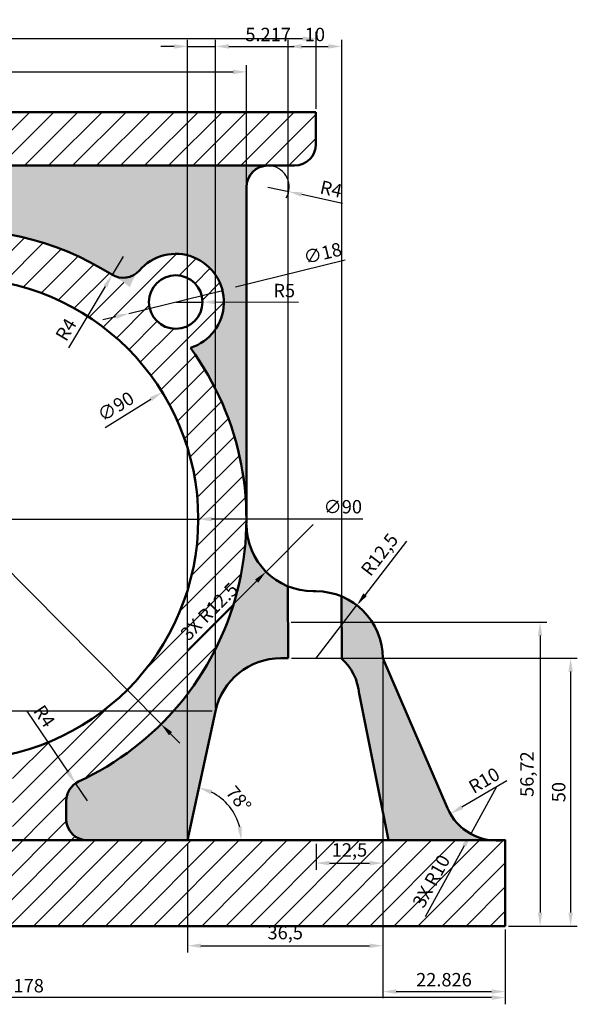
# Model space of a CAD drawing. Units: millimetres. Extents: x 2530 to 2750, y 1494 to 1677.
# Tile 2 of 2: x 2646 to 2750, y 1494 to 1677. Entities that reach past the tile are written whole.
import ezdxf

# ---------------------------------------------------------------- set-up
doc = ezdxf.new("R2010")
doc.units = ezdxf.units.MM
for name, color, linetype, lineweight in [('M-DIMS', 2, 'Continuous', 25), ('M-HATC', 8, 'Continuous', 18), ('M-OUTL', 7, 'Continuous', 50)]:
    doc.layers.add(name, color=color, linetype=linetype, lineweight=lineweight)
doc.styles.get("Standard").update_dxf_attribs({"font": 'arial.ttf'})
doc.dimstyles.new('ISO-25', dxfattribs={"dimtxt": 2.5, "dimasz": 2.5, "dimexe": 1.25, "dimexo": 0.625, "dimtad": 1, "dimtxsty": 'Standard', "dimcen": 2.5, "dimadec": 0, "dimazin": 0, "dimtfac": 1, "dimtmove": 0, "dimatfit": 3, "dimfxl": 1, "dimarcsym": 0})

# ---------------------------------------------------------------- blocks, each defined once
blk = doc.blocks.new('*D3')
at = {"layer": 'Defpoints', "color": 0, "transparency": 16777216}
for p in [(2688.41, 1667.62), (2580.41, 1646.13), (2688.41, 1646.13)]:
    blk.add_point(p, dxfattribs=at)
at = {"layer": 'M-DIMS', "color": 0, "lineweight": -2, "transparency": 16777216}
for p, q in [((2580.41, 1646.75), (2580.41, 1668.87)), ((2688.41, 1646.75), (2688.41, 1668.87)), ((2582.91, 1667.62), (2685.91, 1667.62))]:
    blk.add_line(p, q, dxfattribs=at)
at = {"layer": 'M-DIMS', "color": 0, "transparency": 16777216}
for points in [[(2582.91, 1668.04), (2582.91, 1667.2), (2580.41, 1667.62)], [(2685.91, 1668.04), (2685.91, 1667.2), (2688.41, 1667.62)]]:
    blk.add_solid(points, dxfattribs=at)
at = {"layer": 'M-DIMS', "color": 0, "transparency": 16777216, "insert": (2634.41, 1669.52), "char_height": 2.5, "attachment_point": 5}
blk.add_mtext('108', dxfattribs=at)
blk = doc.blocks.new('*D4')
at = {"layer": 'Defpoints', "color": 0, "transparency": 16777216}
for p in [(2701.41, 1673.83), (2567.41, 1660.13), (2701.41, 1660.13)]:
    blk.add_point(p, dxfattribs=at)
at = {"layer": 'M-DIMS', "color": 0, "lineweight": -2, "transparency": 16777216}
for p, q in [((2567.41, 1660.75), (2567.41, 1675.08)), ((2701.41, 1660.75), (2701.41, 1675.08)), ((2569.91, 1673.83), (2698.91, 1673.83))]:
    blk.add_line(p, q, dxfattribs=at)
at = {"layer": 'M-DIMS', "color": 0, "transparency": 16777216}
for points in [[(2569.91, 1674.25), (2569.91, 1673.41), (2567.41, 1673.83)], [(2698.91, 1674.25), (2698.91, 1673.41), (2701.41, 1673.83)]]:
    blk.add_solid(points, dxfattribs=at)
at = {"layer": 'M-DIMS', "color": 0, "transparency": 16777216, "insert": (2634.41, 1675.73), "char_height": 2.5, "attachment_point": 5}
blk.add_mtext('134', dxfattribs=at)
blk = doc.blocks.new('*D11')
at = {"layer": 'Defpoints', "color": 0, "transparency": 16777216}
for p in [(2677.41, 1524.13), (2713.91, 1524.13), (2713.91, 1504.45)]:
    blk.add_point(p, dxfattribs=at)
at = {"layer": 'M-DIMS', "color": 0, "lineweight": -2, "transparency": 16777216}
for p, q in [((2677.41, 1523.5), (2677.41, 1503.2)), ((2713.91, 1523.5), (2713.91, 1503.2)), ((2679.91, 1504.45), (2711.41, 1504.45))]:
    blk.add_line(p, q, dxfattribs=at)
at = {"layer": 'M-DIMS', "color": 0, "transparency": 16777216}
for points in [[(2679.91, 1504.86), (2679.91, 1504.03), (2677.41, 1504.45)], [(2711.41, 1504.86), (2711.41, 1504.03), (2713.91, 1504.45)]]:
    blk.add_solid(points, dxfattribs=at)
at = {"layer": 'M-DIMS', "color": 0, "transparency": 16777216, "insert": (2695.66, 1506.57), "char_height": 2.5, "attachment_point": 5}
blk.add_mtext('36,5', dxfattribs=at)
blk = doc.blocks.new('*D12')
at = {"layer": 'Defpoints', "color": 0, "transparency": 16777216}
for p in [(2696.18, 1564.85), (2736.73, 1508.13), (2743.28, 1508.13)]:
    blk.add_point(p, dxfattribs=at)
at = {"layer": 'M-DIMS', "color": 0, "lineweight": -2, "transparency": 16777216}
for p, q in [((2696.8, 1564.85), (2744.53, 1564.85)), ((2743.28, 1562.35), (2743.28, 1510.63)), ((2737.36, 1508.13), (2744.53, 1508.13))]:
    blk.add_line(p, q, dxfattribs=at)
at = {"layer": 'M-DIMS', "color": 0, "transparency": 16777216}
for points in [[(2742.86, 1562.35), (2743.69, 1562.35), (2743.28, 1564.85)], [(2742.86, 1510.63), (2743.69, 1510.63), (2743.28, 1508.13)]]:
    blk.add_solid(points, dxfattribs=at)
at = {"layer": 'M-DIMS', "color": 0, "transparency": 16777216, "insert": (2741.15, 1536.49), "char_height": 2.5, "attachment_point": 5, "rotation": 90}
blk.add_mtext('56,72', dxfattribs=at)
blk = doc.blocks.new('*D13')
at = {"layer": 'Defpoints', "color": 0, "transparency": 16777216}
for p in [(2682.63, 1548.27), (2686.45, 1528.53), (2677.41, 1524.13), (2677.41, 1524.13), (2701.41, 1524.13)]:
    blk.add_point(p, dxfattribs=at)
at = {"layer": 'M-DIMS', "color": 0, "lineweight": -2, "transparency": 16777216}
blk.add_arc((2677.41, 1524.13), 10.05, 14.2844, 63.521, dxfattribs=at)
at = {"layer": 'M-DIMS', "color": 0, "transparency": 16777216}
for points in [[(2681.75, 1532.73), (2682.03, 1533.52), (2679.53, 1533.96)], [(2687.56, 1526.66), (2686.74, 1526.56), (2687.46, 1524.13)]]:
    blk.add_solid(points, dxfattribs=at)
at = {"layer": 'M-DIMS', "color": 0, "transparency": 16777216, "insert": (2686.71, 1531.64), "char_height": 2.5, "attachment_point": 5, "rotation": 308.9027}
blk.add_mtext('78°', dxfattribs=at)
blk = doc.blocks.new('*D14')
at = {"layer": 'Defpoints', "color": 0, "transparency": 16777216}
for p in [(2558.73, 1508.13), (2736.73, 1508.13), (2558.73, 1494.76)]:
    blk.add_point(p, dxfattribs=at)
at = {"layer": 'M-DIMS', "color": 0, "lineweight": -2, "transparency": 16777216}
for p, q in [((2558.73, 1507.5), (2558.73, 1493.51)), ((2736.73, 1507.5), (2736.73, 1493.51)), ((2734.23, 1494.76), (2561.23, 1494.76))]:
    blk.add_line(p, q, dxfattribs=at)
at = {"layer": 'M-DIMS', "color": 0, "transparency": 16777216}
for points in [[(2561.23, 1495.17), (2561.23, 1494.34), (2558.73, 1494.76)], [(2734.23, 1495.17), (2734.23, 1494.34), (2736.73, 1494.76)]]:
    blk.add_solid(points, dxfattribs=at)
at = {"layer": 'M-DIMS', "color": 0, "transparency": 16777216, "insert": (2647.73, 1496.66), "char_height": 2.5, "attachment_point": 5}
blk.add_mtext('178', dxfattribs=at)
blk = doc.blocks.new('*D15')
at = {"layer": 'Defpoints', "color": 0, "transparency": 16777216}
for p in [(2701.41, 1524.13), (2713.91, 1524.13), (2713.91, 1519.88)]:
    blk.add_point(p, dxfattribs=at)
at = {"layer": 'M-DIMS', "color": 0, "lineweight": -2, "transparency": 16777216}
for p, q in [((2701.41, 1523.5), (2701.41, 1518.63)), ((2713.91, 1523.5), (2713.91, 1518.63)), ((2703.91, 1519.88), (2711.41, 1519.88))]:
    blk.add_line(p, q, dxfattribs=at)
at = {"layer": 'M-DIMS', "color": 0, "transparency": 16777216}
for points in [[(2703.91, 1520.29), (2703.91, 1519.46), (2701.41, 1519.88)], [(2711.41, 1520.29), (2711.41, 1519.46), (2713.91, 1519.88)]]:
    blk.add_solid(points, dxfattribs=at)
at = {"layer": 'M-DIMS', "color": 0, "transparency": 16777216, "insert": (2707.66, 1522.01), "char_height": 2.5, "attachment_point": 5}
blk.add_mtext('12,5', dxfattribs=at)
blk = doc.blocks.new('*D16')
at = {"layer": 'Defpoints', "color": 0, "transparency": 16777216}
for p in [(2656.49, 1534.79), (2658.73, 1531.48)]:
    blk.add_point(p, dxfattribs=at)
at = {"layer": 'M-DIMS', "color": 0, "lineweight": -2, "transparency": 16777216}
for p, q in [((2647.36, 1548.26), (2655.09, 1536.86)), ((2658.73, 1531.48), (2656.49, 1534.79))]:
    blk.add_line(p, q, dxfattribs=at)
at = {"layer": 'M-DIMS', "color": 0, "transparency": 16777216}
blk.add_solid([(2655.43, 1537.09), (2654.74, 1536.62), (2656.49, 1534.79)], dxfattribs=at)
at = {"layer": 'M-DIMS', "color": 0, "transparency": 16777216, "insert": (2650.39, 1547.13), "char_height": 2.5, "attachment_point": 5, "rotation": 304.1346}
blk.add_mtext('R4', dxfattribs=at)
blk = doc.blocks.new('*D18')
at = {"layer": 'Defpoints', "color": 0, "transparency": 16777216}
for p in [(2735.15, 1534.09), (2726.5, 1529.07)]:
    blk.add_point(p, dxfattribs=at)
at = {"layer": 'M-DIMS', "color": 0, "lineweight": -2, "transparency": 16777216}
blk.add_line((2737.07, 1535.21), (2728.67, 1530.33), dxfattribs=at)
at = {"layer": 'M-DIMS', "color": 0, "transparency": 16777216}
blk.add_solid([(2728.46, 1530.69), (2728.88, 1529.97), (2726.5, 1529.07)], dxfattribs=at)
at = {"layer": 'M-DIMS', "color": 0, "transparency": 16777216, "insert": (2732.99, 1535.04), "char_height": 2.5, "attachment_point": 5, "rotation": 30.1358}
blk.add_mtext('R10', dxfattribs=at)
blk = doc.blocks.new('*D19')
at = {"layer": 'Defpoints', "color": 0, "transparency": 16777216}
for p in [(2709.05, 1568.02), (2701.41, 1558.13)]:
    blk.add_point(p, dxfattribs=at)
at = {"layer": 'M-DIMS', "color": 0, "lineweight": -2, "transparency": 16777216}
for p, q in [((2718.31, 1580.02), (2710.58, 1570)), ((2701.41, 1558.13), (2709.05, 1568.02))]:
    blk.add_line(p, q, dxfattribs=at)
at = {"layer": 'M-DIMS', "color": 0, "transparency": 16777216}
blk.add_solid([(2710.25, 1570.25), (2710.91, 1569.75), (2709.05, 1568.02)], dxfattribs=at)
at = {"layer": 'M-DIMS', "color": 0, "transparency": 16777216, "insert": (2713.53, 1577.3), "char_height": 2.5, "attachment_point": 5, "rotation": 52.3176}
blk.add_mtext('R12,5', dxfattribs=at)
blk = doc.blocks.new('*D20')
at = {"layer": 'Defpoints', "color": 0, "transparency": 16777216}
for p in [(2675.2, 1624.65), (2680.2, 1624.63)]:
    blk.add_point(p, dxfattribs=at)
at = {"layer": 'M-DIMS', "color": 0, "lineweight": -2, "transparency": 16777216}
for p, q in [((2675.2, 1624.65), (2680.2, 1624.63)), ((2698.11, 1624.57), (2682.7, 1624.62))]:
    blk.add_line(p, q, dxfattribs=at)
at = {"layer": 'M-DIMS', "color": 0, "transparency": 16777216}
blk.add_solid([(2682.71, 1625.04), (2682.7, 1624.21), (2680.2, 1624.63)], dxfattribs=at)
at = {"layer": 'M-DIMS', "color": 0, "transparency": 16777216, "insert": (2695.47, 1626.47), "char_height": 2.5, "attachment_point": 5, "rotation": 359.789}
blk.add_mtext('R5', dxfattribs=at)
blk = doc.blocks.new('*D21')
at = {"layer": 'Defpoints', "color": 0, "transparency": 16777216}
for p in [(2683.94, 1626.8), (2666.46, 1622.5)]:
    blk.add_point(p, dxfattribs=at)
at = {"layer": 'M-DIMS', "color": 0, "lineweight": -2, "transparency": 16777216}
for p, q in [((2706.87, 1632.44), (2686.37, 1627.4)), ((2666.46, 1622.5), (2683.94, 1626.8)), ((2664.04, 1621.9), (2661.61, 1621.31))]:
    blk.add_line(p, q, dxfattribs=at)
at = {"layer": 'M-DIMS', "color": 0, "transparency": 16777216}
for points in [[(2686.27, 1627.8), (2686.47, 1626.99), (2683.94, 1626.8)], [(2663.94, 1622.31), (2664.14, 1621.5), (2666.46, 1622.5)]]:
    blk.add_solid(points, dxfattribs=at)
at = {"layer": 'M-DIMS', "color": 0, "transparency": 16777216, "insert": (2702.73, 1633.45), "char_height": 2.5, "attachment_point": 5, "rotation": 13.8127}
blk.add_mtext('∅18', dxfattribs=at)
blk = doc.blocks.new('*D22')
at = {"layer": 'Defpoints', "color": 0, "transparency": 16777216}
for p in [(2692.41, 1646.13), (2696.31, 1645.26)]:
    blk.add_point(p, dxfattribs=at)
at = {"layer": 'M-DIMS', "color": 0, "lineweight": -2, "transparency": 16777216}
for p, q in [((2692.41, 1646.13), (2696.31, 1645.26)), ((2706.34, 1643.03), (2698.75, 1644.72))]:
    blk.add_line(p, q, dxfattribs=at)
blk.add_arc((2692.41, 1646.13), 4, 329.5643, 81.0475, dxfattribs=at)
at = {"layer": 'M-DIMS', "color": 0, "transparency": 16777216}
blk.add_solid([(2698.84, 1645.13), (2698.66, 1644.31), (2696.31, 1645.26)], dxfattribs=at)
at = {"layer": 'M-DIMS', "color": 0, "transparency": 16777216, "insert": (2704.17, 1645.43), "char_height": 2.5, "attachment_point": 5, "rotation": 347.4692}
blk.add_mtext('R4', dxfattribs=at)
blk = doc.blocks.new('*D23')
at = {"layer": 'Defpoints', "color": 0, "transparency": 16777216}
for p in [(2665.38, 1633.17), (2663.34, 1629.73)]:
    blk.add_point(p, dxfattribs=at)
at = {"layer": 'M-DIMS', "color": 0, "lineweight": -2, "transparency": 16777216}
for p, q in [((2665.38, 1633.17), (2663.34, 1629.73)), ((2655.23, 1616.12), (2662.06, 1627.58))]:
    blk.add_line(p, q, dxfattribs=at)
at = {"layer": 'M-DIMS', "color": 0, "transparency": 16777216}
blk.add_solid([(2661.7, 1627.79), (2662.41, 1627.37), (2663.34, 1629.73)], dxfattribs=at)
at = {"layer": 'M-DIMS', "color": 0, "transparency": 16777216, "insert": (2654.97, 1619.34), "char_height": 2.5, "attachment_point": 5, "rotation": 59.2248}
blk.add_mtext('R4', dxfattribs=at)
blk = doc.blocks.new('*D25')
at = {"layer": 'Defpoints', "color": 0, "transparency": 16777216}
for p in [(2672.67, 1607.82), (2596.15, 1560.44)]:
    blk.add_point(p, dxfattribs=at)
at = {"layer": 'M-DIMS', "color": 0, "lineweight": -2, "transparency": 16777216}
blk.add_line((2662, 1601.22), (2670.54, 1606.5), dxfattribs=at)
at = {"layer": 'M-DIMS', "color": 0, "transparency": 16777216}
blk.add_solid([(2670.32, 1606.86), (2670.76, 1606.15), (2672.67, 1607.82)], dxfattribs=at)
at = {"layer": 'M-DIMS', "color": 0, "transparency": 16777216, "insert": (2664.17, 1604.88), "char_height": 2.5, "attachment_point": 5, "rotation": 31.768}
blk.add_mtext('∅90', dxfattribs=at)
blk = doc.blocks.new('*D26')
at = {"layer": 'Defpoints', "color": 0, "transparency": 16777216}
for p in [(2593.48, 1619.36), (2675.33, 1548.9)]:
    blk.add_point(p, dxfattribs=at)
at = {"layer": 'M-DIMS', "color": 0, "lineweight": -2, "transparency": 16777216}
blk.add_line((2615.7, 1600.23), (2595.38, 1617.73), dxfattribs=at)
at = {"layer": 'M-DIMS', "color": 0, "transparency": 16777216}
blk.add_solid([(2595.65, 1618.04), (2595.11, 1617.41), (2593.48, 1619.36)], dxfattribs=at)
at = {"layer": 'M-DIMS', "color": 0, "transparency": 16777216, "insert": (2613.39, 1604.82), "char_height": 2.5, "attachment_point": 5, "rotation": 319.2753}
blk.add_mtext('∅108', dxfattribs=at)
blk = doc.blocks.new('*D29')
at = {"layer": 'Defpoints', "color": 0, "transparency": 16777216}
for p in [(2713.91, 1558.13), (2736.73, 1508.13), (2736.73, 1495.88)]:
    blk.add_point(p, dxfattribs=at)
at = {"layer": 'M-DIMS', "color": 0, "lineweight": -2, "transparency": 16777216}
for p, q in [((2713.91, 1557.5), (2713.91, 1494.63)), ((2736.73, 1507.5), (2736.73, 1494.63)), ((2716.41, 1495.88), (2734.23, 1495.88))]:
    blk.add_line(p, q, dxfattribs=at)
at = {"layer": 'M-DIMS', "color": 0, "transparency": 16777216}
for points in [[(2716.41, 1496.3), (2716.41, 1495.46), (2713.91, 1495.88)], [(2734.23, 1496.3), (2734.23, 1495.46), (2736.73, 1495.88)]]:
    blk.add_solid(points, dxfattribs=at)
at = {"layer": 'M-DIMS', "color": 0, "transparency": 16777216, "insert": (2725.32, 1497.78), "char_height": 2.5, "attachment_point": 5}
blk.add_mtext('22.826', dxfattribs=at)
blk = doc.blocks.new('*D30')
at = {"layer": 'Defpoints', "color": 0, "transparency": 16777216}
for p in [(2696.21, 1558.13), (2736.73, 1508.13), (2748.98, 1508.13)]:
    blk.add_point(p, dxfattribs=at)
at = {"layer": 'M-DIMS', "color": 0, "lineweight": -2, "transparency": 16777216}
for p, q in [((2696.84, 1558.13), (2750.23, 1558.13)), ((2748.98, 1555.63), (2748.98, 1510.63)), ((2737.36, 1508.13), (2750.23, 1508.13))]:
    blk.add_line(p, q, dxfattribs=at)
at = {"layer": 'M-DIMS', "color": 0, "transparency": 16777216}
for points in [[(2748.57, 1555.63), (2749.4, 1555.63), (2748.98, 1558.13)], [(2748.57, 1510.63), (2749.4, 1510.63), (2748.98, 1508.13)]]:
    blk.add_solid(points, dxfattribs=at)
at = {"layer": 'M-DIMS', "color": 0, "transparency": 16777216, "insert": (2747.08, 1533.13), "char_height": 2.5, "attachment_point": 5, "rotation": 90}
blk.add_mtext('50', dxfattribs=at)
blk = doc.blocks.new('*D34')
at = {"layer": 'Defpoints', "color": 0, "transparency": 16777216}
for p in [(2706.21, 1672.38), (2696.21, 1558.13), (2706.21, 1558.15)]:
    blk.add_point(p, dxfattribs=at)
at = {"layer": 'M-DIMS', "color": 0, "lineweight": -2, "transparency": 16777216}
for p, q in [((2696.21, 1558.75), (2696.21, 1673.63)), ((2706.21, 1558.78), (2706.21, 1673.63)), ((2698.71, 1672.38), (2703.71, 1672.38))]:
    blk.add_line(p, q, dxfattribs=at)
at = {"layer": 'M-DIMS', "color": 0, "transparency": 16777216}
for points in [[(2698.71, 1672.8), (2698.71, 1671.96), (2696.21, 1672.38)], [(2703.71, 1672.8), (2703.71, 1671.96), (2706.21, 1672.38)]]:
    blk.add_solid(points, dxfattribs=at)
at = {"layer": 'M-DIMS', "color": 0, "transparency": 16777216, "insert": (2701.21, 1674.28), "char_height": 2.5, "attachment_point": 5}
blk.add_mtext('10', dxfattribs=at)
blk = doc.blocks.new('*D35')
at = {"layer": 'Defpoints', "color": 0, "transparency": 16777216}
for p in [(2682.63, 1672.38), (2682.63, 1548.27), (2677.41, 1524.13)]:
    blk.add_point(p, dxfattribs=at)
at = {"layer": 'M-DIMS', "color": 0, "lineweight": -2, "transparency": 16777216}
for p, q in [((2677.41, 1524.75), (2677.41, 1673.63)), ((2682.63, 1548.89), (2682.63, 1673.63)), ((2674.91, 1672.38), (2672.41, 1672.38)), ((2677.41, 1672.38), (2682.63, 1672.38)), ((2685.13, 1672.38), (2697.31, 1672.38))]:
    blk.add_line(p, q, dxfattribs=at)
at = {"layer": 'M-DIMS', "color": 0, "transparency": 16777216}
for points in [[(2674.91, 1672.8), (2674.91, 1671.96), (2677.41, 1672.38)], [(2685.13, 1672.8), (2685.13, 1671.96), (2682.63, 1672.38)]]:
    blk.add_solid(points, dxfattribs=at)
at = {"layer": 'M-DIMS', "color": 0, "transparency": 16777216, "insert": (2692.47, 1674.28), "char_height": 2.5, "attachment_point": 5}
blk.add_mtext('5.217', dxfattribs=at)
blk = doc.blocks.new('*D36')
at = {"layer": 'Defpoints', "color": 0, "transparency": 16777216}
for p in [(2546.48, 1548.27), (2682.63, 1548.27), (2677.41, 1524.13)]:
    blk.add_point(p, dxfattribs=at)
at = {"layer": 'M-DIMS', "color": 0, "lineweight": -2, "transparency": 16777216}
for p, q in [((2682, 1548.27), (2545.23, 1548.27)), ((2546.48, 1526.63), (2546.48, 1545.77)), ((2676.78, 1524.13), (2545.23, 1524.13))]:
    blk.add_line(p, q, dxfattribs=at)
at = {"layer": 'M-DIMS', "color": 0, "transparency": 16777216}
for points in [[(2546.07, 1545.77), (2546.9, 1545.77), (2546.48, 1548.27)], [(2546.07, 1526.63), (2546.9, 1526.63), (2546.48, 1524.13)]]:
    blk.add_solid(points, dxfattribs=at)
at = {"layer": 'M-DIMS', "color": 0, "transparency": 16777216, "insert": (2544.6, 1536.2), "char_height": 2.5, "attachment_point": 5, "rotation": 90}
blk.add_mtext('24.14', dxfattribs=at)
blk = doc.blocks.new('*D39')
at = {"layer": 'Defpoints', "color": 0, "transparency": 16777216}
for p in [(2596.35, 1622.44), (2672.46, 1545.82)]:
    blk.add_point(p, dxfattribs=at)
at = {"layer": 'M-DIMS', "color": 0, "lineweight": -2, "transparency": 16777216}
for p, q in [((2570.17, 1648.8), (2594.59, 1624.22)), ((2672.46, 1545.82), (2596.35, 1622.44)), ((2674.22, 1544.04), (2675.99, 1542.27))]:
    blk.add_line(p, q, dxfattribs=at)
at = {"layer": 'M-DIMS', "color": 0, "transparency": 16777216}
for points in [[(2594.89, 1624.51), (2594.3, 1623.92), (2596.35, 1622.44)], [(2674.52, 1544.34), (2673.93, 1543.75), (2672.46, 1545.82)]]:
    blk.add_solid(points, dxfattribs=at)
at = {"layer": 'M-DIMS', "color": 0, "transparency": 16777216, "insert": (2574.92, 1646.82), "char_height": 2.5, "attachment_point": 5, "rotation": 314.806}
blk.add_mtext('∅108', dxfattribs=at)
blk = doc.blocks.new('*D40')
at = {"layer": 'Defpoints', "color": 0, "transparency": 16777216}
for p in [(2589.41, 1584.13), (2679.41, 1584.13)]:
    blk.add_point(p, dxfattribs=at)
at = {"layer": 'M-DIMS', "color": 0, "lineweight": -2, "transparency": 16777216}
for p, q in [((2586.91, 1584.13), (2584.41, 1584.13)), ((2589.41, 1584.13), (2679.41, 1584.13)), ((2710.18, 1584.13), (2681.91, 1584.13))]:
    blk.add_line(p, q, dxfattribs=at)
at = {"layer": 'M-DIMS', "color": 0, "transparency": 16777216}
for points in [[(2586.91, 1584.55), (2586.91, 1583.71), (2589.41, 1584.13)], [(2681.91, 1584.55), (2681.91, 1583.71), (2679.41, 1584.13)]]:
    blk.add_solid(points, dxfattribs=at)
at = {"layer": 'M-DIMS', "color": 0, "transparency": 16777216, "insert": (2706.41, 1586.1), "char_height": 2.5, "attachment_point": 5, "rotation": 0.0001}
blk.add_mtext('∅90', dxfattribs=at)
blk = doc.blocks.new('*D44')
at = {"layer": 'Defpoints', "color": 0, "transparency": 16777216}
for p in [(2735.15, 1534.09), (2730.34, 1525.33)]:
    blk.add_point(p, dxfattribs=at)
at = {"layer": 'M-DIMS', "color": 0, "lineweight": -2, "transparency": 16777216}
for p, q in [((2735.15, 1534.09), (2730.34, 1525.33)), ((2721.87, 1509.92), (2729.13, 1523.14))]:
    blk.add_line(p, q, dxfattribs=at)
at = {"layer": 'M-DIMS', "color": 0, "transparency": 16777216}
blk.add_solid([(2728.77, 1523.34), (2729.5, 1522.94), (2730.34, 1525.33)], dxfattribs=at)
at = {"layer": 'M-DIMS', "color": 0, "transparency": 16777216, "insert": (2723.23, 1516.35), "char_height": 2.5, "attachment_point": 5, "rotation": 61.2066}
blk.add_mtext('3X R10', dxfattribs=at)
blk = doc.blocks.new('*D45')
at = {"layer": 'Defpoints', "color": 0, "transparency": 16777216}
for p in [(2700.91, 1583.13), (2692.07, 1574.29)]:
    blk.add_point(p, dxfattribs=at)
at = {"layer": 'M-DIMS', "color": 0, "lineweight": -2, "transparency": 16777216}
for p, q in [((2700.91, 1583.13), (2692.07, 1574.29)), ((2677.55, 1559.79), (2690.3, 1572.53))]:
    blk.add_line(p, q, dxfattribs=at)
at = {"layer": 'M-DIMS', "color": 0, "transparency": 16777216}
blk.add_solid([(2690, 1572.82), (2690.59, 1572.23), (2692.07, 1574.29)], dxfattribs=at)
at = {"layer": 'M-DIMS', "color": 0, "transparency": 16777216, "insert": (2681.69, 1566.62), "char_height": 2.5, "attachment_point": 5, "rotation": 44.9767}
blk.add_mtext('3X R12.5', dxfattribs=at)

msp = doc.modelspace()

# ---------------------------------------------------------------- hatches: boundary and pattern name
at = {"layer": 'M-HATC'}
h = msp.add_hatch(dxfattribs=at)
h.set_pattern_fill('ANSI31', color=256)
h.paths.add_polyline_path([(2701.4085, 1660.1289), (2688.4085, 1660.1289), (2567.4085, 1660.1289), (2567.4085, 1654.1289, 0.41421356), (2571.4085, 1650.1289), (2580.4085, 1650.1289), (2688.4085, 1650.1289), (2697.4085, 1650.1289, 0.41421356), (2701.4085, 1654.1289)])
h.paths.add_polyline_path([(2679.4085, 1584.1289, -0.34791599), (2644.7344, 1540.3297), (2644.7344, 1524.1289), (2654.7344, 1524.1289), (2658.7344, 1524.1289, -0.41421356), (2654.7344, 1528.1289), (2654.7344, 1531.4768, -0.29243225), (2657.0568, 1535.108, 0.47416598), (2677.944, 1616.0767, 1.63457651), (2666.6504, 1627.447, 0.86114512), (2590.873, 1552.1812, 1.31927608), (2600.4123, 1537.7124, -0.37066508), (2605.5707, 1538.4739, 0.03574325), (2612.3671, 1534.8321, -0.29578567), (2614.7344, 1531.1805), (2614.7344, 1524.1289), (2624.7344, 1524.1289), (2624.7344, 1540.1811, -0.14401207), (2602.4811, 1552.4171), (2597.1599, 1547.1318, -0.19803221), (2598.6124, 1543.6082, -1), (2588.6124, 1543.6082, -0.6694042), (2597.1599, 1547.1318), (2602.4811, 1552.4171, -0.19803221), (2589.4085, 1584.1289, -1)])
h.paths.add_polyline_path([(2680.2046, 1624.6496, -1), (2670.2046, 1624.6496, -1)], flags=16)
h.paths.add_polyline_path([(2736.7344, 1524.1289), (2735.977, 1524.1289, -0.04128859), (2734.3283, 1524.1289), (2577.9283, 1524.1289, -0.03968429), (2576.3434, 1524.1289), (2558.7344, 1524.1289), (2558.7344, 1508.1289), (2736.7344, 1508.1289)])
h = msp.add_hatch(color=256, dxfattribs=at)
h.dxf.hatch_style = 1
h.paths.add_polyline_path([(2688.4085, 1646.1289, -0.41421356), (2692.4085, 1650.1289), (2688.4085, 1650.1289), (2580.4085, 1650.1289), (2576.4085, 1650.1289, -0.41421356), (2580.4085, 1646.1289), (2580.4085, 1584.1289, -0.61677219), (2666.6504, 1627.447, -1.63457651), (2677.944, 1616.0767, -0.15960296), (2688.4085, 1584.1289)])
h.paths.add_polyline_path([(2696.1494, 1571.5708, -0.30814487), (2688.4024, 1583.3173, -0.28835772), (2657.0568, 1535.108, 0.29243225), (2654.7344, 1531.4768), (2654.7344, 1528.1289, 0.41421356), (2658.7344, 1524.1289), (2677.4085, 1524.1289), (2682.6254, 1548.2693, -0.35316368), (2694.8434, 1558.1289), (2696.2102, 1558.1289)])
h.paths.add_polyline_path([(2713.9085, 1558.1289, 0.30415201), (2706.158, 1569.6915), (2706.2106, 1558.0572, -0.18754445), (2709.4561, 1551.5776), (2714.9622, 1524.1289), (2734.3283, 1524.1289, -0.27714511), (2725.9689, 1530.1379)])
h.paths.add_polyline_path([(2614.7344, 1531.1805, 0.29578567), (2612.3671, 1534.8321, -0.03574325), (2605.5707, 1538.4739, 0.37066508), (2600.4123, 1537.7124, -0.512533), (2585.8599, 1539.0368), (2585.8445, 1539.0127, -0.54802528), (2577.9283, 1524.1289), (2614.7344, 1524.1289)])

# ---------------------------------------------------------------- linework, layer by layer
at = {"layer": 'M-OUTL'}
for p, q in [((2567.4085, 1660.1289), (2688.4085, 1660.1289)), ((2688.4085, 1660.1289), (2701.4085, 1660.1289)), ((2701.4085, 1660.1289), (2701.4085, 1654.1289)), ((2580.4085, 1650.1289), (2688.4085, 1650.1289)), ((2697.4085, 1650.1289), (2688.4085, 1650.1289)), ((2688.4085, 1646.1289), (2688.4085, 1584.1289)), ((2696.1494, 1571.5708), (2696.2102, 1558.1289)), ((2701.4085, 1570.6289), (2700.8988, 1570.6293)), ((2706.158, 1569.6915), (2706.2103, 1558.1289)), ((2696.2102, 1558.1289), (2694.8434, 1558.1289)), ((2706.1064, 1558.1502), (2706.2102, 1558.1507)), ((2706.2103, 1558.1289), (2706.1304, 1558.1289)), ((2713.9085, 1558.1289), (2725.9689, 1530.1379)), ((2714.9622, 1524.1289), (2709.4644, 1551.536)), ((2709.4662, 1551.4632), (2709.4784, 1551.4663)), ((2677.4085, 1524.1289), (2682.6254, 1548.2693)), ((2654.7344, 1528.1289), (2654.7344, 1531.4768)), ((2558.7344, 1524.1289), (2736.7344, 1524.1289)), ((2644.7344, 1524.1289), (2654.7344, 1524.1289)), ((2701.4085, 1524.1289), (2677.4085, 1524.1289)), ((2701.4085, 1524.1289), (2713.9085, 1524.1289)), ((2736.7344, 1508.1289), (2736.7344, 1524.2208)), ((2736.7344, 1508.1289), (2736.7344, 1524.1289)), ((2558.7344, 1508.1289), (2736.7344, 1508.1289))]:
    msp.add_line(p, q, dxfattribs=at)
for centre, radius in [((2634.4085, 1584.1289), 45), ((2675.2046, 1624.6496), 5)]:
    msp.add_circle(centre, radius, dxfattribs=at)
for centre, radius, start, end in [((2697.4085, 1654.1289), 4, 270, 0), ((2692.4085, 1646.1289), 4, 90, 180), ((2634.4085, 1584.1289), 54, 57.721584, 211.89027), ((2675.2046, 1624.6496), 9, 287.720787, 139.073521), ((2665.3825, 1633.1658), 4, 237.721584, 319.073521), ((2634.4085, 1584.1289), 54, 294.797512, 36.272378), ((2700.9085, 1583.1293), 12.5, 180, 269.955726), ((2701.4085, 1558.1289), 12.5, 0, 90), ((2694.8434, 1545.6289), 12.5, 90, 167.805483), ((2699.4998, 1550.6433), 10, 4.702852, 48.650068), ((2658.7344, 1531.4768), 4, 114.797512, 180), ((2735.1527, 1534.0949), 10, 203.309551, 279.101035), ((2658.7344, 1528.1289), 4, 180, 270)]:
    msp.add_arc(centre, radius, start, end, dxfattribs=at)

# ---------------------------------------------------------------- dimensions: what is measured, and where the dimension line sits
at = {"layer": 'M-DIMS'}
for base, p1, p2, override, picture, middle in [((2701.4085, 1673.8298), (2567.4085, 1660.1289), (2701.4085, 1660.1289), {"dimclrd": 0, "dimclre": 0, "dimclrt": 0}, '*D4', (2634.4085, 1675.7321)), ((2682.6254, 1672.3789), (2677.4085, 1524.1289), (2682.6254, 1548.2693), {"dimdec": 3, "dimlfac": 1, "dimrnd": 0, "dimzin": 0, "dimdsep": 46, "dimlunit": 2}, '*D35', (2692.4685, 1674.2804)), ((2706.2102, 1672.3789), (2696.2102, 1558.1289), (2706.2102, 1558.1507), {"dimdec": 0, "dimlfac": 1, "dimrnd": 0, "dimzin": 0, "dimdsep": 46, "dimlunit": 2}, '*D34', (2701.2102, 1674.2804)), ((2688.4085, 1667.6183), (2580.4085, 1646.1289), (2688.4085, 1646.1289), {"dimclrd": 0, "dimclre": 0, "dimclrt": 0}, '*D3', (2634.4085, 1669.5198)), ((2736.7344, 1495.8789), (2713.9085, 1558.1289), (2736.7344, 1508.1289), {"dimdec": 3, "dimlfac": 1, "dimrnd": 0, "dimzin": 0, "dimdsep": 46, "dimlunit": 2}, '*D29', (2725.3215, 1497.7804)), ((2713.9085, 1504.4472), (2677.4085, 1524.1289), (2713.9085, 1524.1289), {"dimclrd": 0, "dimclre": 0, "dimclrt": 0}, '*D11', (2695.6585, 1506.5746)), ((2713.9085, 1519.8779), (2701.4085, 1524.1289), (2713.9085, 1524.1289), {"dimclrd": 0, "dimclre": 0, "dimclrt": 0}, '*D15', (2707.6585, 1522.0053)), ((2558.7344, 1494.7581), (2736.7344, 1508.1289), (2558.7344, 1508.1289), {"dimclrd": 0, "dimclre": 0, "dimclrt": 0}, '*D14', (2647.7344, 1496.6596))]:
    dim = msp.add_linear_dim(base=base, p1=p1, p2=p2, dimstyle='ISO-25', override=override, dxfattribs=at)
    dim.commit()
    dim.dimension.update_dxf_attribs({"geometry": picture, "text_midpoint": middle})
for p1, p2, override, picture, middle in [((2672.4628, 1545.8161), (2596.3542, 1622.4418), {"dimdec": 0, "dimlfac": 1, "dimrnd": 0, "dimzin": 0, "dimdsep": 46, "dimlunit": 2}, '*D39', (2573.5217, 1645.4295)), ((2666.4649, 1622.5009), (2683.9444, 1626.7984), {"dimclrd": 0, "dimclre": 0, "dimclrt": 0}, '*D21', (2703.2024, 1631.5331)), ((2675.3326, 1548.898), (2593.4844, 1619.3599), {"dimclrd": 0, "dimclre": 0, "dimclrt": 0}, '*D26', (2612.1037, 1603.3308)), ((2596.1501, 1560.4373), (2672.6669, 1607.8206), {"dimclrd": 0, "dimclre": 0, "dimclrt": 0}, '*D25', (2665.2096, 1603.2027)), ((2589.4085, 1584.1289), (2679.4085, 1584.129), {"dimdec": 0, "dimlfac": 1, "dimrnd": 0, "dimzin": 0, "dimdsep": 46, "dimlunit": 2}, '*D40', (2706.4085, 1584.129))]:
    dim = msp.add_diameter_dim_2p(p1=p1, p2=p2, dimstyle='ISO-25', override=override, dxfattribs=at)
    dim.commit()
    dim.dimension.update_dxf_attribs({"geometry": picture, "text_midpoint": middle, "dimtype": 163})
for center, mpoint, picture, middle in [((2692.4085, 1646.1289), (2696.3132, 1645.2611), '*D22', (2704.1737, 1645.4348)), ((2701.4085, 1558.1289), (2709.0496, 1568.0216), '*D19', (2713.5262, 1577.2975))]:
    dim = msp.add_radius_dim(center=center, mpoint=mpoint, dimstyle='ISO-25', override={"dimclrd": 0, "dimclre": 0, "dimclrt": 0}, dxfattribs=at)
    dim.commit()
    dim.dimension.update_dxf_attribs({"geometry": picture, "text_midpoint": middle})
for center, mpoint, picture, middle in [((2665.3825, 1633.1658), (2663.3358, 1629.7291), '*D23', (2656.5774, 1618.3807)), ((2675.2046, 1624.6496), (2680.2046, 1624.6312), '*D20', (2695.4638, 1624.575)), ((2658.7344, 1531.4768), (2656.4899, 1534.7877), '*D16', (2648.8359, 1546.0778)), ((2735.1527, 1534.0949), (2726.5043, 1529.0744), '*D18', (2733.9485, 1533.3958))]:
    dim = msp.add_radius_dim(center=center, mpoint=mpoint, dimstyle='ISO-25', override={"dimclrd": 0, "dimclre": 0, "dimclrt": 0}, dxfattribs=at)
    dim.commit()
    dim.dimension.update_dxf_attribs({"geometry": picture, "text_midpoint": middle, "dimtype": 164})
for center, mpoint, override, picture, middle in [((2700.9085, 1583.1293), (2692.0661, 1574.2941), {"dimdec": 1, "dimlfac": 1, "dimrnd": 0, "dimzin": 0, "dimdsep": 46, "dimlunit": 2}, '*D45', (2681.6933, 1566.6189)), ((2735.1527, 1534.0949), (2730.3362, 1525.3313), {"dimdec": 0, "dimlfac": 1, "dimrnd": 0, "dimzin": 0, "dimdsep": 46, "dimlunit": 2}, '*D44', (2723.2299, 1516.3511))]:
    dim = msp.add_radius_dim(center=center, mpoint=mpoint, text='3X <>', dimstyle='ISO-25', override=override, dxfattribs=at)
    dim.commit()
    dim.dimension.update_dxf_attribs({"geometry": picture, "text_midpoint": middle})
for base, p1, p2, override, picture, middle in [((2743.2778, 1508.1289), (2696.1798, 1564.8498), (2736.7344, 1508.1289), {"dimclrd": 0, "dimclre": 0, "dimclrt": 0}, '*D12', (2741.1504, 1536.4894)), ((2748.9844, 1508.1289), (2696.2102, 1558.1289), (2736.7344, 1508.1289), {"dimdec": 0, "dimlfac": 1, "dimrnd": 0, "dimzin": 0, "dimdsep": 46, "dimlunit": 2}, '*D30', (2747.083, 1533.1289)), ((2546.4844, 1548.2693), (2677.4085, 1524.1289), (2682.6254, 1548.2693), {"dimdec": 2, "dimlfac": 1, "dimrnd": 0, "dimzin": 0, "dimdsep": 46, "dimlunit": 2}, '*D36', (2544.6043, 1536.1991))]:
    dim = msp.add_linear_dim(base=base, p1=p1, p2=p2, angle=90, dimstyle='ISO-25', override=override, dxfattribs=at)
    dim.commit()
    dim.dimension.update_dxf_attribs({"geometry": picture, "text_midpoint": middle})
dim = msp.add_angular_dim_2l(base=(2686.4497, 1528.5259), line1=((2701.4085, 1524.1289), (2677.4085, 1524.1289)), line2=((2677.4085, 1524.1289), (2682.6254, 1548.2693)), dimstyle='ISO-25', override={"dimclrd": 0, "dimclre": 0, "dimclrt": 0}, dxfattribs=at)
dim.commit()
dim.dimension.update_dxf_attribs({"geometry": '*D13', "text_midpoint": (2686.7121, 1531.6367)})

doc.saveas('drawing.dxf')
